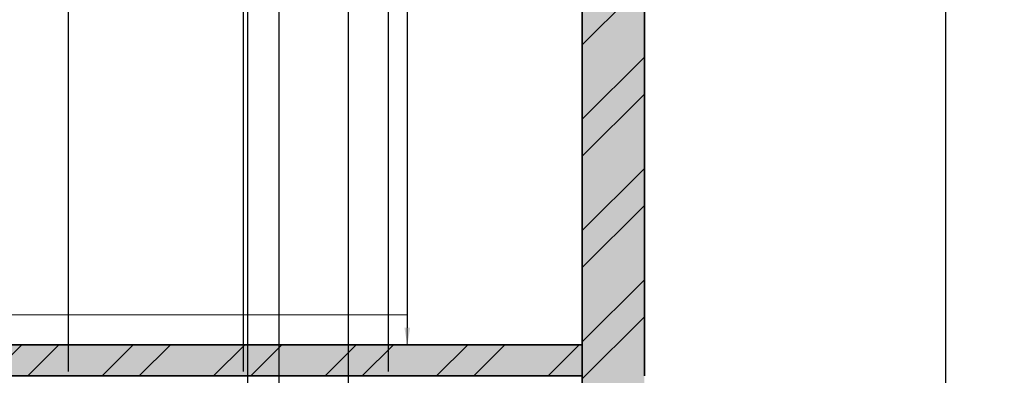
# Model space of a CAD drawing. Units: inches. Extents: x 1804 to 3296, y 909 to 2477.
# Tile 18 of 31: x 2235 to 2378, y 1587 to 1638. Entities that reach past the tile are written whole.
import ezdxf

# ---------------------------------------------------------------- set-up
doc = ezdxf.new("R2010")
doc.units = ezdxf.units.IN
for name, color, linetype, lineweight in [('A-ANNO-DIMS', 2, 'Continuous', 18), ('A-ANNO-TTLB', 156, 'Continuous', 35), ('A-WALL-PATT', 10, 'Continuous', 13), ('FUR', 100, 'Continuous', 18), ('WALL', 10, 'Continuous', 35)]:
    doc.layers.add(name, color=color, linetype=linetype, lineweight=lineweight)
doc.styles.get("Standard").update_dxf_attribs({"font": 'arial.ttf'})
doc.dimstyles.new('ISO-25', dxfattribs={"dimtxt": 5, "dimasz": 2.5, "dimexe": 1.25, "dimexo": 0.625, "dimtad": 1, "dimdec": 0, "dimlunit": 4, "dimtxsty": 'Standard', "dimcen": 2.5, "dimadec": 0, "dimazin": 0, "dimtfac": 1, "dimtdec": 0, "dimtmove": 0, "dimatfit": 3, "dimfxl": 1, "dimarcsym": 0})
pattern_1 = [(45, (0, 196.207), (-8.08223, 8.08223), []), (45, (5.388, 196.207), (-8.08223, 8.08223), [])]

# ---------------------------------------------------------------- blocks, each defined once
blk = doc.blocks.new('*D11')
at = {"layer": 'A-ANNO-DIMS', "color": 0, "lineweight": -2, "transparency": 16777216}
for p, q in [((2315.91, 1784.38), (2289.92, 1784.38)), ((2291.17, 1781.88), (2291.17, 1593.42)), ((2315.91, 1590.92), (2289.92, 1590.92))]:
    blk.add_line(p, q, dxfattribs=at)
at = {"layer": 'A-ANNO-DIMS', "color": 0, "lineweight": 100, "transparency": 16777216}
for points in [[(2290.75, 1781.88), (2291.58, 1781.88), (2291.17, 1784.38)], [(2290.75, 1593.42), (2291.58, 1593.42), (2291.17, 1590.92)]]:
    blk.add_solid(points, dxfattribs=at)
at = {"layer": 'Defpoints', "color": 0, "lineweight": 100, "transparency": 16777216}
for p in [(2316.54, 1784.38), (2291.17, 1590.92), (2316.54, 1590.92)]:
    blk.add_point(p, dxfattribs=at)
at = {"layer": 'A-ANNO-DIMS', "color": 0, "transparency": 16777216, "insert": (2287.99, 1687.65), "char_height": 5, "attachment_point": 5, "rotation": 90}
blk.add_mtext('16\'-1"', dxfattribs=at)
blk = doc.blocks.new('*D53')
at = {"layer": 'A-ANNO-DIMS', "color": 0, "lineweight": -2, "transparency": 16777216}
for p, q in [((2326.16, 1793.38), (2370.49, 1793.38)), ((2369.24, 1140.57), (2369.24, 1790.88)), ((2326.16, 1138.07), (2370.49, 1138.07))]:
    blk.add_line(p, q, dxfattribs=at)
at = {"layer": 'A-ANNO-DIMS', "color": 0, "lineweight": 100, "transparency": 16777216}
for points in [[(2368.82, 1790.88), (2369.65, 1790.88), (2369.24, 1793.38)], [(2368.82, 1140.57), (2369.65, 1140.57), (2369.24, 1138.07)]]:
    blk.add_solid(points, dxfattribs=at)
at = {"layer": 'Defpoints', "color": 0, "lineweight": 100, "transparency": 16777216}
for p in [(2325.54, 1793.38), (2369.24, 1793.38), (2325.54, 1138.07)]:
    blk.add_point(p, dxfattribs=at)
at = {"layer": 'A-ANNO-DIMS', "color": 0, "transparency": 16777216, "insert": (2366.03, 1465.72), "char_height": 5, "attachment_point": 5, "rotation": 90}
blk.add_mtext('54\'-7 1/2"', dxfattribs=at)
blk = doc.blocks.new('*D56')
at = {"layer": 'A-ANNO-DIMS', "color": 0, "lineweight": -2, "transparency": 16777216}
for p, q in [((2180.87, 1680.42), (2180.87, 975.89)), ((2268, 1680.42), (2268, 975.89)), ((2183.37, 977.14), (2265.5, 977.14))]:
    blk.add_line(p, q, dxfattribs=at)
at = {"layer": 'A-ANNO-DIMS', "color": 0, "lineweight": 100, "transparency": 16777216}
for points in [[(2183.37, 977.56), (2183.37, 976.72), (2180.87, 977.14)], [(2265.5, 977.56), (2265.5, 976.72), (2268, 977.14)]]:
    blk.add_solid(points, dxfattribs=at)
at = {"layer": 'Defpoints', "color": 0, "lineweight": 100, "transparency": 16777216}
for p in [(2180.87, 1681.04), (2268, 1681.04), (2268, 977.14)]:
    blk.add_point(p, dxfattribs=at)
at = {"layer": 'A-ANNO-DIMS', "color": 0, "transparency": 16777216, "insert": (2224.44, 980.32), "char_height": 5, "attachment_point": 5}
blk.add_mtext('7\'-3"', dxfattribs=at)
blk = doc.blocks.new('*D65')
at = {"layer": 'A-ANNO-DIMS', "color": 0, "lineweight": -2, "transparency": 16777216}
for p, q in [((2282.65, 1466.57), (2282.65, 1874.99)), ((2316.54, 1466.57), (2316.54, 1874.99)), ((2285.15, 1873.74), (2314.04, 1873.74))]:
    blk.add_line(p, q, dxfattribs=at)
at = {"layer": 'A-ANNO-DIMS', "color": 0, "lineweight": 100, "transparency": 16777216}
for points in [[(2285.15, 1874.15), (2285.15, 1873.32), (2282.65, 1873.74)], [(2314.04, 1874.15), (2314.04, 1873.32), (2316.54, 1873.74)]]:
    blk.add_solid(points, dxfattribs=at)
at = {"layer": 'Defpoints', "color": 0, "lineweight": 100, "transparency": 16777216}
for p in [(2316.54, 1873.74), (2282.65, 1465.94), (2316.54, 1465.94)]:
    blk.add_point(p, dxfattribs=at)
at = {"layer": 'A-ANNO-DIMS', "color": 0, "transparency": 16777216, "insert": (2299.6, 1876.91), "char_height": 5, "attachment_point": 5}
blk.add_mtext('2\'-10"', dxfattribs=at)
blk = doc.blocks.new('*D67')
at = {"layer": 'A-ANNO-DIMS', "color": 0, "lineweight": -2, "transparency": 16777216}
for p, q in [((2267.43, 1587.05), (2267.43, 1874.99)), ((2288.43, 1587.05), (2288.43, 1874.99)), ((2269.93, 1873.74), (2285.93, 1873.74))]:
    blk.add_line(p, q, dxfattribs=at)
at = {"layer": 'A-ANNO-DIMS', "color": 0, "lineweight": 100, "transparency": 16777216}
for points in [[(2269.93, 1874.15), (2269.93, 1873.32), (2267.43, 1873.74)], [(2285.93, 1874.15), (2285.93, 1873.32), (2288.43, 1873.74)]]:
    blk.add_solid(points, dxfattribs=at)
at = {"layer": 'Defpoints', "color": 0, "lineweight": 100, "transparency": 16777216}
for p in [(2288.43, 1873.74), (2267.43, 1586.42), (2288.43, 1586.42)]:
    blk.add_point(p, dxfattribs=at)
at = {"layer": 'A-ANNO-DIMS', "color": 0, "transparency": 16777216, "insert": (2277.93, 1876.91), "char_height": 5, "attachment_point": 5}
blk.add_mtext('1\'-9"', dxfattribs=at)
blk = doc.blocks.new('*D68')
at = {"layer": 'A-ANNO-DIMS', "color": 0, "lineweight": -2, "transparency": 16777216}
for p, q in [((2242.06, 1587.05), (2242.06, 1874.99)), ((2267.43, 1587.05), (2267.43, 1874.99)), ((2244.56, 1873.74), (2264.93, 1873.74)), ((2267.43, 1873.74), (2296.2, 1873.74))]:
    blk.add_line(p, q, dxfattribs=at)
at = {"layer": 'A-ANNO-DIMS', "color": 0, "lineweight": 100, "transparency": 16777216}
for points in [[(2244.56, 1874.15), (2244.56, 1873.32), (2242.06, 1873.74)], [(2264.93, 1874.15), (2264.93, 1873.32), (2267.43, 1873.74)]]:
    blk.add_solid(points, dxfattribs=at)
at = {"layer": 'Defpoints', "color": 0, "lineweight": 100, "transparency": 16777216}
for p in [(2267.43, 1873.74), (2242.06, 1586.42), (2267.43, 1586.42)]:
    blk.add_point(p, dxfattribs=at)
at = {"layer": 'A-ANNO-DIMS', "color": 0, "transparency": 16777216, "insert": (2283.07, 1876.95), "char_height": 5, "attachment_point": 5}
blk.add_mtext('2\'-1 1/2"', dxfattribs=at)
blk = doc.blocks.new('*D73')
at = {"layer": 'A-ANNO-DIMS', "color": 0, "lineweight": -2, "transparency": 16777216}
for p, q in [((2272.59, 1272.26), (2272.59, 1874.99)), ((2316.54, 1272.26), (2316.54, 1874.99)), ((2275.09, 1873.74), (2314.04, 1873.74))]:
    blk.add_line(p, q, dxfattribs=at)
at = {"layer": 'A-ANNO-DIMS', "color": 0, "lineweight": 100, "transparency": 16777216}
for points in [[(2275.09, 1874.15), (2275.09, 1873.32), (2272.59, 1873.74)], [(2314.04, 1874.15), (2314.04, 1873.32), (2316.54, 1873.74)]]:
    blk.add_solid(points, dxfattribs=at)
at = {"layer": 'Defpoints', "color": 0, "lineweight": 100, "transparency": 16777216}
for p in [(2316.54, 1873.74), (2272.59, 1271.63), (2316.54, 1271.63)]:
    blk.add_point(p, dxfattribs=at)
at = {"layer": 'A-ANNO-DIMS', "color": 0, "transparency": 16777216, "insert": (2294.56, 1876.92), "char_height": 5, "attachment_point": 5}
blk.add_mtext('3\'-8"', dxfattribs=at)

msp = doc.modelspace()

# ---------------------------------------------------------------- hatches: boundary and pattern name
at = {"layer": 'A-ANNO-TTLB'}
h = msp.add_hatch(color=256, dxfattribs=at)
h.dxf.hatch_style = 1
h.paths.add_polyline_path([(3294.53, 2476.54), (1803.79, 2476.54), (1805.43, 909.47), (3296.17, 909.47)])
h.paths.add_polyline_path([(1811, 914.33), (1812.79, 2467.54), (3285.53, 2467.54), (3283.74, 914.33)], flags=16)
h.paths.add_polyline_path([(1925.58, 1062.77), (1925.58, 1138.07), (1925.58, 1539.88), (1925.58, 1793.38), (1925.58, 1830.04), (2325.54, 1830.04), (2325.54, 1793.38), (2325.54, 1586.42), (2325.54, 1138.07), (2325.54, 1062.77)], flags=0)
h.paths.add_polyline_path([(1997.22, 1029.4), (2008.85, 1037.96), (2008.85, 1020.84)], flags=0)
h.paths.add_polyline_path([(1934.58, 1138.07), (1934.58, 1147.07), (2078.77, 1147.07), (2078.77, 1138.07), (2060.94, 1138.07)], flags=0)
h.paths.add_polyline_path([(1944.35, 1138.07), (1944.35, 1147.07), (2056.05, 1147.07), (2056.05, 1138.07)], flags=0)
h.paths.add_polyline_path([(2222.24, 1037.96), (2233.87, 1029.4), (2222.24, 1020.84)], flags=0)
h.paths.add_polyline_path([(2061.94, 1139.07), (2061.94, 1146.07), (2077.77, 1146.07), (2077.77, 1139.07)], flags=0)
h.paths.add_polyline_path([(2149.58, 1138.07), (2149.58, 1269.44), (2158.58, 1269.44), (2158.58, 1326.69), (2149.58, 1326.69), (2149.58, 1340.94), (2139.6, 1340.94), (2139.6, 1434.25), (2149.58, 1434.25), (2149.58, 1447.36), (2158.58, 1447.36), (2158.58, 1423.87), (2158.58, 1408.06), (2198.46, 1408.06), (2198.46, 1412.56), (2282.65, 1412.56), (2282.65, 1465.94), (2316.54, 1465.94), (2316.54, 1590.92), (2192.86, 1590.92), (2192.86, 1595.3), (2291.17, 1595.3), (2291.17, 1590.92), (2316.54, 1590.92), (2316.54, 1784.38), (2300.24, 1784.38), (2300.24, 1757.47), (2268, 1757.47), (2268, 1681.04), (2180.87, 1681.04), (2180.87, 1757.47), (2148.63, 1757.47), (2148.63, 1784.38), (2119.08, 1784.38), (2119.08, 1585.58), (2114.58, 1585.58), (2114.58, 1784.38), (2064.11, 1784.38), (2046.28, 1784.38), (2046.28, 1760.38), (1958.58, 1760.38), (1958.58, 1664.38), (1934.58, 1664.38), (1934.58, 1784.38), (1934.58, 1793.38), (2046.28, 1793.38), (2064.11, 1793.38), (2119.08, 1793.38), (2230.78, 1793.38), (2230.78, 1784.38), (2268, 1784.38), (2300.24, 1784.38), (2316.54, 1784.38), (2316.54, 1590.92), (2316.54, 1373.73), (2316.54, 1138.07)], flags=0)
h.paths.add_polyline_path([(2209.19, 1166.63), (2209.19, 1175.63), (2158.58, 1175.63), (2209.19, 1223.63), (2209.19, 1231.63), (2183.88, 1231.63), (2183.88, 1301.66), (2242.59, 1301.66), (2242.59, 1326.69), (2316.54, 1326.69), (2272.59, 1271.63), (2272.59, 1223.63), (2316.54, 1175.63), (2272.59, 1175.63), (2272.59, 1166.63)], flags=0)
h.paths.add_polyline_path([(1947.77, 1345.22), (1947.77, 1457.48), (1991.2, 1457.48), (1991.2, 1451.7), (1991.2, 1352.18), (1991.2, 1345.22)], flags=0)
h.paths.add_polyline_path([(2209.19, 1271.63), (2262.59, 1271.63), (2262.59, 1311.85), (2272.59, 1301.66), (2272.59, 1271.63), (2269.92, 1269.63), (2270.59, 1269.63), (2270.59, 1225.63), (2211.19, 1225.63), (2211.19, 1269.63), (2211.86, 1269.63)], flags=0)
h.paths.add_polyline_path([(2000.34, 1378.21), (2000.34, 1429.71), (2025.22, 1429.71), (2025.22, 1378.21)], flags=0)
h.paths.add_polyline_path([(2001.34, 1379.21), (2001.34, 1428.71), (2024.22, 1428.71), (2024.22, 1379.21)], flags=0)
h.paths.add_polyline_path([(2012.34, 1390.21), (2012.34, 1417.71), (2013.22, 1417.71), (2013.22, 1390.21)], flags=0)
h.paths.add_polyline_path([(2237.56, 1331.19), (2237.56, 1340.18), (2238.62, 1340.18), (2238.62, 1386.84), (2241.04, 1386.84), (2242.06, 1386.84), (2242.06, 1408.06), (2316.54, 1331.19)], flags=0)
h.paths.add_polyline_path([(1953.73, 1464.35), (1953.73, 1498.59), (1981.74, 1498.59), (1981.74, 1464.35)], flags=0)
h.paths.add_polyline_path([(1987.63, 1462.08), (1987.63, 1500.95), (2104.07, 1500.95), (2104.07, 1462.08), (2099.27, 1462.08), (1993.6, 1462.08)], flags=0)
h.paths.add_polyline_path([(1956.06, 1481.47, -1), (1979.41, 1481.47, -1)], flags=0)
edge = h.paths.add_edge_path(flags=0)
edge.add_ellipse((2299.53, 1438.37), major_axis=(0.31, 21.36), ratio=0.670333, start_angle=0, end_angle=360)
h.paths.add_polyline_path([(2297.39, 1438.37, -1), (2301.67, 1438.37, -1)], flags=0)
h.paths.add_polyline_path([(2591.54, 1163.23), (2591.54, 1179.38), (2591.54, 1379.68), (2591.54, 1395.84), (2734.5, 1395.84), (2734.5, 1379.68), (2734.5, 1179.38), (2734.5, 1163.23)], flags=0)
h.paths.add_polyline_path([(2592.54, 1164.23), (2592.54, 1166.23), (2733.5, 1166.23), (2733.5, 1164.23)], flags=0)
h.paths.add_polyline_path([(2592.54, 1180.38), (2592.54, 1378.68), (2733.5, 1378.68), (2733.5, 1180.38)], flags=0)
h.paths.add_polyline_path([(2593.54, 1181.38), (2593.54, 1377.68), (2732.5, 1377.68), (2732.5, 1181.38)], flags=0)
h.paths.add_polyline_path([(2594.54, 1182.38), (2594.54, 1376.68), (2731.5, 1376.68), (2731.5, 1182.38)], flags=0)
h.paths.add_polyline_path([(1936.95, 1697.46), (1936.95, 1736.46), (1955.41, 1736.46), (1955.41, 1697.46)], flags=0)
h.paths.add_polyline_path([(1938.48, 1718.36), (1938.48, 1734.92), (1953.65, 1734.92), (1953.65, 1718.36)], flags=0)
h.paths.add_polyline_path([(1944.75, 1726.64, -1), (1947.37, 1726.64, -1)], flags=0)
h.paths.add_polyline_path([(2592.54, 1394.84), (2733.5, 1394.84), (2733.5, 1392.84), (2592.54, 1392.84)], flags=0)
h.paths.add_polyline_path([(1976.61, 1762.5), (1976.61, 1781.44), (2012.79, 1781.44), (2012.79, 1762.5)], flags=0)
h.paths.add_polyline_path([(1979.57, 1771.97, -1), (1991.39, 1771.97, -1)], flags=0)
h.paths.add_polyline_path([(1995.36, 1771.97, -1), (2007.18, 1771.97, -1)], flags=0)
h.paths.add_polyline_path([(2251.51, 1744.53), (2268, 1730.05), (2251.51, 1730.05)], flags=0)
h.paths.add_polyline_path([(2047.28, 1785.38), (2047.28, 1792.38), (2063.11, 1792.38), (2063.11, 1785.38)], flags=0)
h.paths.add_polyline_path([(2155.08, 1770.92, -1), (2174.42, 1770.92, -1)], flags=0)
h.paths.add_polyline_path([(2188.59, 1758.27), (2188.59, 1772.81), (2222.3, 1772.81), (2222.3, 1758.27)], flags=0)
h.paths.add_polyline_path([(2223.97, 1758.27), (2223.97, 1772.81), (2257.68, 1772.81), (2257.68, 1758.27)], flags=0)
h.paths.add_polyline_path([(2274.45, 1770.92, -1), (2293.8, 1770.92, -1)], flags=0)
h.paths.add_polyline_path([(2591.54, 1582.09), (2591.54, 1782.39), (2734.5, 1782.39), (2734.5, 1582.09)], flags=0)
h.paths.add_polyline_path([(2592.54, 1583.09), (2592.54, 1781.39), (2733.5, 1781.39), (2733.5, 1583.09)], flags=0)
h.paths.add_polyline_path([(2593.54, 1584.09), (2593.54, 1780.39), (2732.5, 1780.39), (2732.5, 1584.09)], flags=0)
h.paths.add_polyline_path([(2594.54, 1585.09), (2594.54, 1779.39), (2731.5, 1779.39), (2731.5, 1585.09)], flags=0)
h.paths.add_polyline_path([(1922.17, 1978.79), (1922.17, 2295.08), (1922.17, 2296.08), (2115.67, 2296.08), (2115.67, 2384.31), (2115.67, 2385.31), (2322.12, 2385.31), (2323.12, 2385.31), (2323.12, 1979.79), (2323.12, 1978.79), (1923.17, 1978.79)], flags=0)
h.paths.add_polyline_path([(1922.17, 1978.79), (1922.17, 2051.31), (1922.17, 2214.86), (1922.17, 2296.08), (2115.67, 2296.08), (2115.67, 2385.31), (2323.12, 2385.31), (2323.12, 2280.42), (2323.12, 1978.79), (2115.67, 1978.79)], flags=0)
h.paths.add_polyline_path([(1923.17, 1979.79), (1923.17, 2050.31), (2115.67, 2050.31), (2115.67, 2051.31), (1923.17, 2051.31), (1923.17, 2213.86), (1923.17, 2214.86), (1923.17, 2295.08), (1990.02, 2295.08), (1990.02, 2214.86), (1991.02, 2214.86), (1991.02, 2295.08), (2115.67, 2295.08), (2115.67, 1979.79), (2116.67, 1979.79), (2116.67, 2304.18), (2116.67, 2384.31), (2322.12, 2384.31), (2322.12, 2280.42), (2322.12, 1979.79), (2115.67, 1979.79)], flags=0)
h.paths.add_polyline_path([(2972.46, 1192.5), (2972.46, 1196.92), (2995.47, 1196.92), (2995.47, 1255.47), (2995.09, 1255.47), (2987.42, 1249.39), (2980.08, 1255.47), (2978.05, 1255.47), (2978.05, 1257.24), (2995.47, 1257.24), (2995.47, 1261.58), (3015.37, 1261.58), (3015.37, 1333.28), (3015.37, 1414.4), (3032.82, 1414.4), (3032.82, 1333.28), (3032.82, 1261.58), (3052.66, 1261.58), (3052.66, 1255.47), (3079.86, 1255.47), (3078.72, 1254.57), (3081.47, 1252.29), (3078.56, 1249.99), (3075.81, 1252.26), (3072.57, 1249.69), (3070.36, 1251.52), (3067.67, 1249.39), (3060.34, 1255.47), (3052.66, 1255.47), (3052.66, 1196.92), (3054.58, 1196.92), (3074, 1196.92), (3074, 1192.5), (3052.66, 1192.5), (2995.47, 1192.5)], flags=0)
h.paths.add_polyline_path([(2490.75, 1979.27), (2490.75, 1980.27), (2596.87, 1980.27), (2596.87, 2051.8), (2596.87, 2052.8), (2596.87, 2216.35), (2596.87, 2297.57), (2717.32, 2297.57), (2710.57, 2305.62), (2724.07, 2305.62), (2717.32, 2297.57), (2782.37, 2297.57), (2782.37, 2395.8), (3006.82, 2395.8), (3006.82, 1981.27), (3093.73, 1981.27), (3093.73, 1980.27), (3047.51, 1980.27), (3046.37, 1979.37), (3049.11, 1977.1), (3046.2, 1974.79), (3043.46, 1977.07), (3040.21, 1974.49), (3038, 1976.32), (3035.32, 1974.2), (3027.98, 1980.27), (2871.83, 1980.27), (2871.83, 1981.27), (2791.37, 1981.27), (2791.37, 2050.8), (2597.87, 2050.8), (2597.87, 1980.27), (2597.87, 1979.27), (2546.27, 1979.27), (2545.12, 1978.37), (2547.87, 1976.1), (2544.96, 1973.79), (2542.22, 1976.07), (2538.97, 1973.49), (2536.76, 1975.32), (2534.07, 1973.2), (2526.74, 1979.27)], flags=0)
h.paths.add_polyline_path([(2597.87, 2051.8), (2606.87, 2051.8), (2606.87, 2258.39), (2597.87, 2258.39), (2597.87, 2296.57), (2606.87, 2296.57), (2606.87, 2262.39), (2782.37, 2262.39), (2782.37, 2296.57), (2790.37, 2296.57), (2790.37, 2262.39), (2791.37, 2262.39), (2791.37, 2305.67), (2791.37, 2385.8), (2996.82, 2385.8), (2996.82, 2339.85), (3006.82, 2339.85), (3006.82, 2250.12), (2997.82, 2250.12), (2997.82, 1981.27), (2996.82, 1981.27), (2872.83, 1981.27), (2872.83, 1991.8), (2871.83, 1991.8), (2871.83, 2050.8), (2790.37, 2050.8), (2597.87, 2050.8)], flags=0)
h.paths.add_polyline_path([(2179.93, 2153.92), (2179.93, 2353.97), (2259.98, 2353.97), (2259.98, 2153.92)], flags=0)
h.paths.add_polyline_path([(2180.93, 2154.92), (2180.93, 2352.97), (2258.98, 2352.97), (2258.98, 2154.92)], flags=0)
h.paths.add_polyline_path([(2960.87, 1608.49), (2960.87, 1753.62), (3070.9, 1753.62), (3070.9, 1608.49)], flags=0)
h.paths.add_polyline_path([(2961.87, 1609.49), (2961.87, 1752.62), (3069.9, 1752.62), (3069.9, 1609.49)], flags=0)
h.paths.add_polyline_path([(2962.87, 1610.49), (2962.87, 1751.62), (3068.9, 1751.62), (3068.9, 1610.49)], flags=0)
h.paths.add_polyline_path([(2963.87, 1611.49), (2963.87, 1750.62), (3067.9, 1750.62), (3067.9, 1611.49)], flags=0)
h.paths.add_polyline_path([(2782.37, 2051.8), (2782.37, 2216.32), (2791.37, 2216.32), (2791.37, 2051.8), (2872.83, 2051.8), (2872.83, 2068.56), (2884.67, 2068.56), (2884.67, 2085.33), (2896.51, 2085.33), (2896.51, 2102.09), (2908.36, 2102.09), (2908.36, 2118.85), (2920.2, 2118.85), (2920.2, 2135.62), (2932.05, 2135.62), (2932.05, 2145.3), (2925.08, 2145.3), (2925.08, 2203.2), (2996.82, 2203.2), (2996.82, 2145.3), (2953.82, 2145.3), (2872.83, 2051.8), (2790.37, 2051.8)], flags=0)
h.paths.add_polyline_path([(2717.32, 2238.65), (2710.57, 2246.7), (2724.07, 2246.7)], flags=0)
h.paths.add_polyline_path([(2003.09, 1122.79), (2017.16, 1122.79), (2017.16, 1138.74), (2003.09, 1138.74)], flags=8)
h.paths.add_polyline_path([(2174.76, 1792.72), (2188.83, 1792.72), (2188.83, 1808.66), (2174.76, 1808.66)], flags=8)
h.paths.add_polyline_path([(1987.95, 1792.51), (2002.02, 1792.51), (2002.02, 1808.45), (1987.95, 1808.45)], flags=8)
h.paths.add_polyline_path([(2148.79, 1289.26), (2160.46, 1289.26), (2160.46, 1305.2), (2148.79, 1305.2)], flags=8)
h.paths.add_polyline_path([(2115.36, 1133.57), (2127.04, 1133.57), (2127.04, 1149.51), (2115.36, 1149.51)], flags=8)
h.paths.add_polyline_path([(2237.58, 1421.48), (2249.25, 1421.48), (2249.25, 1437.43), (2237.58, 1437.43)], flags=8)
h.paths.add_polyline_path([(2134.99, 1584.32), (2146.66, 1584.32), (2146.66, 1600.26), (2134.99, 1600.26)], flags=8)
h.paths.add_polyline_path([(2101.95, 1557.31), (2113.62, 1557.31), (2113.62, 1573.25), (2101.95, 1573.25)], flags=8)
h.paths.add_polyline_path([(2937.85, 1156.77), (3120.41, 1156.77), (3120.41, 1185.72), (2937.85, 1185.72)], flags=8)
h.paths.add_polyline_path([(2980.71, 1786.71), (3050.06, 1786.71), (3050.06, 1802.66), (2980.71, 1802.66)], flags=8)
h.paths.add_polyline_path([(2869.28, 1661.96), (2938.62, 1661.96), (2938.62, 1690.8), (2869.28, 1690.8)], flags=8)
h.paths.add_polyline_path([(3092.27, 1674.86), (3161.62, 1674.86), (3161.62, 1690.8), (3092.27, 1690.8)], flags=8)
h.paths.add_polyline_path([(2980.71, 1674.86), (3050.06, 1674.86), (3050.06, 1690.8), (2980.71, 1690.8)], flags=8)
h.paths.add_polyline_path([(2649.07, 1678.23), (2674.53, 1678.23), (2674.53, 1714.76), (2649.07, 1714.76)], flags=8)
h.paths.add_polyline_path([(2530.84, 1981.63), (2549.13, 1981.63), (2549.13, 1997.57), (2530.84, 1997.57)], flags=8)
h.paths.add_polyline_path([(3031.29, 1981.77), (3049.58, 1981.77), (3049.58, 1997.71), (3031.29, 1997.71)], flags=8)
h.paths.add_polyline_path([(2715.38, 1911.9), (2851.54, 1911.9), (2851.54, 1940.85), (2715.38, 1940.85)], flags=8)
h.paths.add_polyline_path([(2015.23, 1927.36), (2205.42, 1927.36), (2205.42, 1956.3), (2015.23, 1956.3)], flags=8)
h.paths.add_polyline_path([(2671.84, 2057.84), (2702.75, 2057.84), (2702.75, 2073.79), (2671.84, 2073.79)], flags=8)
h.paths.add_polyline_path([(2678.5, 2316.52), (2765.26, 2316.52), (2765.26, 2332.46), (2678.5, 2332.46)], flags=8)
h.paths.add_polyline_path([(2678.48, 2271.96), (2736.41, 2271.96), (2736.41, 2287.9), (2678.48, 2287.9)], flags=8)
h.paths.add_polyline_path([(2019.2, 972.79), (2243.21, 972.79), (2243.21, 1001.74), (2019.2, 1001.74)], flags=8)
h.paths.add_polyline_path([(2097.06, 1021.56), (2132.16, 1021.56), (2132.16, 1037.51), (2097.06, 1037.51)], flags=8)
h.paths.add_polyline_path([(2182.47, 1360.48), (2207.35, 1360.48), (2207.35, 1376.42), (2182.47, 1376.42)], flags=8)
h.paths.add_polyline_path([(2261.12, 1361.77), (2295.01, 1361.77), (2295.01, 1377.71), (2261.12, 1377.71)], flags=8)
h.paths.add_polyline_path([(2245.75, 1511.51), (2278.44, 1511.51), (2278.44, 1527.46), (2245.75, 1527.46)], flags=8)
h.paths.add_polyline_path([(1991.16, 1296.29), (2060.51, 1296.29), (2060.51, 1312.23), (1991.16, 1312.23)], flags=8)
h.paths.add_polyline_path([(2187, 1651.35), (2246.71, 1651.35), (2246.71, 1667.29), (2187, 1667.29)], flags=8)
h.paths.add_polyline_path([(1976.49, 1684.81), (2068.63, 1684.81), (2068.63, 1700.76), (1976.49, 1700.76)], flags=8)
at = {"layer": 'A-WALL-PATT'}
h = msp.add_hatch(dxfattribs=at)
h.set_pattern_fill('ANSI32', color=256, scale=1.2)
h.set_pattern_definition(pattern_1)
h.paths.add_polyline_path([(1934.58, 1784.38), (1934.58, 1793.38), (1925.58, 1793.38), (1925.58, 1539.88), (2119.08, 1539.88), (2119.08, 1545.58), (2114.58, 1545.58), (2114.58, 1544.38), (1934.58, 1544.38)])
h.paths.add_polyline_path([(2114.58, 1793.38), (2064.11, 1793.38), (2064.11, 1784.38), (2114.58, 1784.38)], flags=17)
h.paths.add_polyline_path([(2325.54, 1793.38), (2230.78, 1793.38), (2230.78, 1784.38), (2268, 1784.38), (2300.24, 1784.38), (2316.54, 1784.38), (2316.54, 1590.92), (2316.54, 1586.42), (2325.54, 1586.42)])
h.paths.add_polyline_path([(1944.35, 1147.07), (1934.58, 1147.07), (1934.58, 1138.07), (1944.35, 1138.07)])
h.paths.add_polyline_path([(2101.21, 1144.07, -0.01877), (2101.32, 1147.07), (2078.77, 1147.07), (2078.77, 1138.07), (2101.21, 1138.07)])
h.paths.add_polyline_path([(1934.58, 1539.88), (1925.58, 1539.88), (1925.58, 1138.07), (1934.58, 1138.07), (1934.58, 1147.07)])
h.paths.add_polyline_path([(2325.54, 1586.42), (2316.54, 1586.42), (2316.54, 1373.73), (2316.54, 1138.07), (2325.54, 1138.07), (2325.54, 1228.97)])
h.paths.add_polyline_path([(2158.58, 1423.87), (2158.58, 1447.36), (2149.58, 1447.36), (2149.58, 1423.87), (2149.58, 1340.94), (2149.58, 1326.69), (2158.58, 1326.69), (2158.58, 1354.23), (2158.58, 1402.2)])
h.paths.add_polyline_path([(2316.54, 1412.56), (2282.65, 1412.56), (2273.09, 1412.56), (2273.09, 1408.06), (2316.54, 1408.06)])
h.paths.add_polyline_path([(2273.09, 1412.56), (2242.06, 1412.56), (2242.06, 1408.06), (2273.09, 1408.06)])
h.paths.add_polyline_path([(2237.56, 1412.56), (2198.46, 1412.56), (2198.46, 1408.06), (2237.56, 1408.06)])
h.paths.add_polyline_path([(2242.06, 1408.06), (2237.56, 1408.06), (2237.56, 1386.84), (2242.06, 1386.84)])
h.paths.add_polyline_path([(2242.06, 1412.56), (2237.56, 1412.56), (2237.56, 1408.06), (2242.06, 1408.06)])
h.paths.add_polyline_path([(2158.58, 1269.44), (2149.58, 1269.44), (2149.58, 1138.07), (2158.58, 1138.07)])
h.paths.add_polyline_path([(2149.58, 1147.07), (2141.21, 1147.07), (2141.21, 1144.07), (2141.21, 1138.07), (2149.58, 1138.07)])
h.paths.add_polyline_path([(2272.59, 1175.63), (2209.19, 1175.63), (2209.19, 1166.63), (2272.59, 1166.63)])
h.paths.add_polyline_path([(2237.56, 1446.21), (2242.06, 1446.21), (2242.06, 1586.42), (2237.56, 1586.42)])
h.paths.add_polyline_path([(2242.06, 1414.58), (2237.56, 1414.58), (2237.56, 1412.56), (2242.06, 1412.56)])
h = msp.add_hatch(color=256, dxfattribs=at)
h.dxf.hatch_style = 1
h.paths.add_polyline_path([(2114.58, 1793.38), (2064.11, 1793.38), (2064.11, 1784.38), (2114.58, 1784.38)])
h.paths.add_polyline_path([(2119.08, 1793.38), (2114.58, 1793.38), (2114.58, 1585.58), (2119.08, 1585.58)])
h.paths.add_polyline_path([(2325.54, 1793.38), (2230.78, 1793.38), (2230.78, 1784.38), (2268, 1784.38), (2316.54, 1784.38), (2316.54, 1590.92), (2316.54, 1586.42), (2325.54, 1586.42)])
h.paths.add_polyline_path([(2316.54, 1331.19), (2158.58, 1331.19), (2158.58, 1326.69), (2316.54, 1326.69)])
h.paths.add_polyline_path([(2242.06, 1408.06), (2237.56, 1408.06), (2237.56, 1386.84), (2242.06, 1386.84)])
h.paths.add_polyline_path([(2242.06, 1412.56), (2237.56, 1412.56), (2237.56, 1408.06), (2242.06, 1408.06)])
h.paths.add_polyline_path([(2237.56, 1412.56), (2198.46, 1412.56), (2198.46, 1408.06), (2237.56, 1408.06)])
h.paths.add_polyline_path([(2273.09, 1412.56), (2242.06, 1412.56), (2242.06, 1408.06), (2273.09, 1408.06)])
h.paths.add_polyline_path([(2316.54, 1412.56), (2282.65, 1412.56), (2273.09, 1412.56), (2273.09, 1408.06), (2316.54, 1408.06)])
h.paths.add_polyline_path([(2325.54, 1586.42), (2316.54, 1586.42), (2316.54, 1373.73), (2316.54, 1138.07), (2325.54, 1138.07), (2325.54, 1228.97)])
h.paths.add_polyline_path([(2272.59, 1175.63), (2209.19, 1175.63), (2209.19, 1166.63), (2272.59, 1166.63)])
h = msp.add_hatch(dxfattribs=at)
h.set_pattern_fill('ANSI32', color=256, scale=1.2)
h.set_pattern_definition(pattern_1)
h.paths.add_polyline_path([(2161.83, 1590.92), (2161.83, 1586.42), (2316.54, 1586.42), (2316.54, 1590.92)])
h = msp.add_hatch(color=256, dxfattribs=at)
h.dxf.hatch_style = 1
h.paths.add_polyline_path([(2316.54, 1590.92), (2161.83, 1590.92), (2161.83, 1586.42), (2316.54, 1586.42)])

# ---------------------------------------------------------------- linework, layer by layer
at = {"layer": 'FUR'}
msp.add_lwpolyline([(2192.86, 1590.92), (2291.17, 1590.92), (2291.17, 1595.3), (2192.86, 1595.3)], close=True, dxfattribs=at)
at = {"layer": 'WALL'}
for p, q in [((2325.54, 1793.38), (2325.54, 1586.42)), ((2316.54, 1784.38), (2316.54, 1590.92)), ((2316.54, 1590.92), (2161.83, 1590.92)), ((2316.54, 1590.92), (2316.54, 1373.73))]:
    msp.add_line(p, q, dxfattribs=at)
msp.add_lwpolyline([(2161.83, 1586.42), (2316.54, 1586.42), (2316.54, 1590.92), (2161.83, 1590.92)], close=True, dxfattribs=at)

# ---------------------------------------------------------------- dimensions: what is measured, and where the dimension line sits
at = {"layer": 'A-ANNO-DIMS'}
for base, p1, p2, picture, middle in [((2267.43, 1873.74), (2242.06, 1586.42), (2267.43, 1586.42), '*D68', (2283.07, 1876.95)), ((2288.43, 1873.74), (2267.43, 1586.42), (2288.43, 1586.42), '*D67', (2277.93, 1876.91)), ((2316.5375, 1873.7362), (2272.5886, 1271.6342), (2316.5375, 1271.6342), '*D73', (2294.563, 1876.9158)), ((2316.54, 1873.74), (2282.65, 1465.94), (2316.54, 1465.94), '*D65', (2299.6, 1876.91)), ((2268, 977.14), (2180.87, 1681.04), (2268, 1681.04), '*D56', (2224.44, 980.32))]:
    dim = msp.add_linear_dim(base=base, p1=p1, p2=p2, dimstyle='ISO-25', override={"dimdec": 1, "dimlfac": 1, "dimrnd": 0, "dimzin": 1, "dimdsep": 46, "dimlunit": 4, "dimfrac": 2}, dxfattribs=at)
    dim.commit()
    dim.dimension.update_dxf_attribs({"geometry": picture, "text_midpoint": middle})
for base, p1, p2, override, picture, middle in [((2369.24, 1793.38), (2325.54, 1138.07), (2325.54, 1793.38), {"dimdec": 1, "dimlfac": 1, "dimrnd": 0, "dimzin": 1, "dimdsep": 46, "dimlunit": 4, "dimfrac": 2}, '*D53', (2366.03, 1465.72)), ((2291.17, 1590.92), (2316.54, 1784.38), (2316.54, 1590.92), {"dimclrd": 0, "dimclre": 0, "dimclrt": 0}, '*D11', (2287.99, 1687.65))]:
    dim = msp.add_linear_dim(base=base, p1=p1, p2=p2, angle=90, dimstyle='ISO-25', override=override, dxfattribs=at)
    dim.commit()
    dim.dimension.update_dxf_attribs({"geometry": picture, "text_midpoint": middle})

doc.saveas('drawing.dxf')
